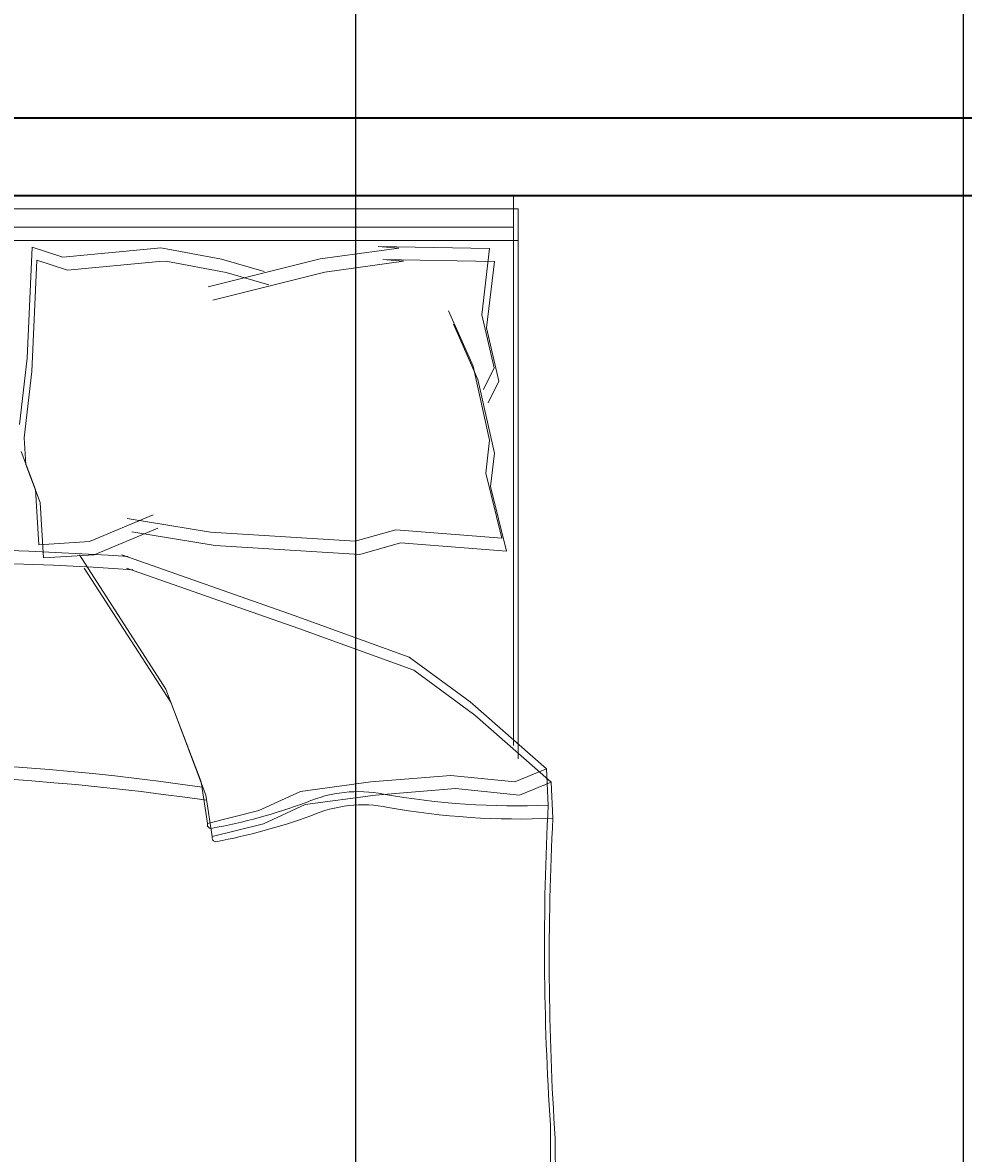
# Model space of a CAD drawing. Units: inches. Extents: x 1088 to 1703, y 668 to 1875.
# Tile 43 of 45: x 1531 to 1586, y 1743 to 1809. Entities that reach past the tile are written whole.
import ezdxf

# ---------------------------------------------------------------- set-up
doc = ezdxf.new("R2010")
doc.units = ezdxf.units.IN
for name, color, linetype, lineweight in [('A-ANNO-DIMS', 2, 'Continuous', 18), ('A-FURN', 8, 'Continuous', 13), ('A-WALL', 7, 'Continuous', 35)]:
    doc.layers.add(name, color=color, linetype=linetype, lineweight=lineweight)
doc.styles.get("Standard").update_dxf_attribs({"font": 'arial.ttf'})
doc.dimstyles.get("Standard").update_dxf_attribs({"dimtxt": 0.18, "dimasz": 0.18, "dimexe": 0.18, "dimexo": 0.0625, "dimgap": 0.09, "dimtad": 0, "dimtih": 1, "dimtoh": 1, "dimdec": 4, "dimzin": 0, "dimdsep": 46, "dimtxsty": 'Standard', "dimcen": 0.09, "dimadec": 0, "dimazin": 0, "dimtfac": 1, "dimtdec": 4, "dimtofl": 0, "dimtmove": 0, "dimatfit": 3, "dimfxl": 1, "dimtolj": 1, "dimtzin": 0, "dimarcsym": 0})

# ---------------------------------------------------------------- blocks, each defined once
blk = doc.blocks.new('BED-DOUBLE')
for p, q in [((34.03, 63.655), (30.133, 59.213)), ((36.121, 63.75), (34.03, 63.655, 4.641)), ((34.772, 61.812), (34.03, 63.655)), ((33.263, 63.381), (29.367, 58.939)), ((35.355, 63.476), (33.263, 63.381, 4.641)), ((34.006, 61.538), (33.263, 63.381)), ((0.766, 61.734), (32.668, 61.734)), ((0.766, 4.44), (0.766, 61.734)), ((2.605, 4.44), (2.605, 61.734)), ((34.401, 58.099), (34.772, 61.812)), ((0, 61.46), (31.901, 61.46)), ((0, 4.167), (0, 61.46)), ((1.838, 4.167), (1.838, 61.46)), ((20.635, 61.054), (16.872, 60.124)), ((20.151, 54.902), (20.635, 61.054)), ((33.634, 57.825), (34.006, 61.538)), ((3.832, 60.351), (3.716, 53.875)), ((3.832, 60.351), (7.681, 59.897)), ((7.681, 59.897), (10.763, 60.611)), ((14.947, 60.351), (10.665, 59.389)), ((10.763, 60.611), (12.017, 59.995)), ((16.872, 60.124), (14.947, 60.351)), ((19.868, 60.78), (16.105, 59.851)), ((19.384, 54.628), (19.868, 60.78)), ((3.065, 60.077), (2.949, 53.601)), ((3.065, 60.077), (6.915, 59.624)), ((6.915, 59.624), (9.996, 60.337)), ((14.181, 60.078), (9.899, 59.115)), ((9.996, 60.337), (11.251, 59.721)), ((16.105, 59.851), (14.181, 60.078)), ((9.899, 59.115), (6.688, 57.699)), ((10.665, 59.389), (7.454, 57.973)), ((30.133, 59.213), (27.535, 55.685)), ((29.367, 58.939), (26.769, 55.411)), ((34.006, 53.183), (33.634, 57.825)), ((34.772, 53.457), (34.401, 58.099)), ((26.769, 55.411), (24.357, 48.727)), ((27.535, 55.685), (25.123, 49.001)), ((2.949, 53.601), (3.048, 54.803)), ((3.048, 54.803), (3.68, 50.25)), ((3.716, 53.875), (3.814, 55.077)), ((3.814, 55.077), (4.446, 50.523)), ((20.052, 52.278), (19.384, 54.628)), ((20.819, 52.552), (20.151, 54.902)), ((34.562, 49.098), (34.006, 53.183)), ((35.329, 49.372), (34.772, 53.457)), ((20.302, 44.148), (20.819, 52.552)), ((19.536, 43.874), (20.052, 52.278)), ((4.446, 50.523), (6.068, 44.027)), ((3.68, 50.25), (5.301, 43.753)), ((36.442, 46.958), (35.329, 49.372)), ((24.357, 48.727), (20.84, 38.731)), ((25.123, 49.001), (21.606, 39.005)), ((35.676, 46.685), (34.562, 49.098)), ((5.171, 47.27), (4.457, 44.794)), ((4.404, 46.996), (3.69, 44.52)), ((36.418, 43.714), (35.676, 46.685)), ((37.184, 43.988), (36.442, 46.958)), ((4.457, 44.794), (3.808, 41.281)), ((3.69, 44.52), (3.042, 41.007)), ((19.503, 39.314), (20.302, 44.148)), ((34.772, 43.616), (37.184, 43.988)), ((18.736, 39.04), (19.536, 43.874)), ((28.624, 41.3), (34.006, 43.342)), ((29.391, 41.574), (34.772, 43.616)), ((34.006, 43.342), (36.418, 43.714)), ((21.606, 36.551), (29.391, 41.574)), ((3.042, 41.007), (3.066, 40.622)), ((3.808, 41.281), (3.832, 40.896)), ((3.832, 40.896), (4.338, 35.587)), ((20.835, 37.139), (19.294, 40.82)), ((20.84, 36.277), (28.624, 41.3)), ((3.066, 40.622), (3.571, 35.314)), ((20.068, 36.866), (18.528, 40.547)), ((20.252, 33.925), (20.068, 36.866)), ((21.018, 34.199), (20.835, 37.139)), ((4.338, 35.587), (3.754, 33.814)), ((3.571, 35.314), (2.987, 33.541)), ((17.81, 33.998), (21.018, 34.199)), ((2.987, 33.541), (9.432, 33.249)), ((3.754, 33.814), (10.198, 33.523)), ((10.198, 33.523), (14.047, 33.069)), ((14.838, 32.892), (17.044, 33.725)), ((15.604, 33.166), (17.81, 33.998)), ((17.044, 33.725), (20.252, 33.925)), ((9.432, 33.249), (13.281, 32.795)), ((14.047, 33.069), (15.604, 33.166))]:
    blk.add_line(p, q)
for centre, radius, start, end in [((-7.213, 61.808), 43.378, 349.87628, 2.56571), ((44.303, 218.785), 155.251, 266.97912, 273.83645), ((81.308, -5405.342), 5469.019, 90.002168, 90.286887), ((82.075, -5405.068), 5469.019, 90.002168, 90.286887), ((-7.98, 61.534), 43.378, 349.87628, 2.56571), ((43.537, 218.511), 155.251, 266.97912, 273.83645), ((42.039, 52.443), 7.462, 168.6608, 203.73842), ((42.806, 52.716), 7.462, 168.6608, 203.73842), ((1.777, 37.349), 35.551, 10.66171, 19.88058), ((2.543, 37.623), 35.551, 10.66171, 19.88058), ((37.259, 44.196), 0.221, 250.24637, 1.13765), ((187.401, 21.287), 154.676, 171.78449, 186.90062), ((188.167, 21.561), 154.676, 171.78449, 186.90062), ((36.492, 43.922), 0.221, 250.24637, 1.13765), ((219.021, 25.88), 197.774, 176.08655, 186.78213), ((218.255, 25.607), 197.774, 176.08655, 186.78213)]:
    blk.add_arc(centre, radius, start, end)
blk = doc.blocks.new('*D28')
at = {"layer": 'A-ANNO-DIMS', "color": 0, "lineweight": -2, "transparency": 16777216}
for p, q in [((1170.345, 1803.621), (1170.345, 1857.788)), ((1170.525, 1857.608), (1408.147, 1857.608)), ((1646.563, 1857.608), (1408.941, 1857.608)), ((1646.743, 1745.552), (1646.743, 1857.788))]:
    blk.add_line(p, q, dxfattribs=at)
at = {"layer": 'A-ANNO-DIMS', "color": 0, "transparency": 16777216}
for points in [[(1170.525, 1857.638), (1170.525, 1857.578), (1170.345, 1857.608)], [(1646.563, 1857.638), (1646.563, 1857.578), (1646.743, 1857.608)]]:
    blk.add_solid(points, dxfattribs=at)
at = {"layer": 'Defpoints', "color": 0, "transparency": 16777216}
for p in [(1646.743, 1857.608), (1170.345, 1803.558), (1646.743, 1745.49)]:
    blk.add_point(p, dxfattribs=at)
at = {"layer": 'A-ANNO-DIMS', "color": 0, "transparency": 16777216, "insert": (1408.544, 1857.608), "char_height": 0.18, "attachment_point": 5}
blk.add_mtext('\\A1;476.4', dxfattribs=at)
blk = doc.blocks.new('*D32')
at = {"layer": 'A-ANNO-DIMS', "color": 0, "lineweight": -2, "transparency": 16777216}
for p, q in [((1550.595, 1373.121), (1550.595, 1857.788)), ((1550.775, 1857.608), (1567.825, 1857.608)), ((1585.665, 1857.608), (1568.614, 1857.608)), ((1585.845, 1360.983), (1585.845, 1857.788))]:
    blk.add_line(p, q, dxfattribs=at)
at = {"layer": 'A-ANNO-DIMS', "color": 0, "transparency": 16777216}
for points in [[(1550.775, 1857.638), (1550.775, 1857.578), (1550.595, 1857.608)], [(1585.665, 1857.638), (1585.665, 1857.578), (1585.845, 1857.608)]]:
    blk.add_solid(points, dxfattribs=at)
at = {"layer": 'Defpoints', "color": 0, "transparency": 16777216}
for p in [(1585.845, 1857.608), (1550.595, 1373.058), (1585.845, 1360.921)]:
    blk.add_point(p, dxfattribs=at)
at = {"layer": 'A-ANNO-DIMS', "color": 0, "transparency": 16777216, "insert": (1568.22, 1857.608), "char_height": 0.18, "attachment_point": 5}
blk.add_mtext('\\A1;35.25', dxfattribs=at)

msp = doc.modelspace()

# ---------------------------------------------------------------- linework, layer by layer
at = {"layer": 'A-WALL'}
for p, q in [((1437.345, 1803.558), (1624.845, 1803.558)), ((1437.345, 1803.558), (1624.845, 1803.558)), ((1437.345, 1803.558), (1624.845, 1803.558)), ((1437.345, 1803.558), (1624.845, 1803.558)), ((1437.345, 1803.558), (1624.845, 1803.558)), ((1441.845, 1799.058), (1620.345, 1799.058))]:
    msp.add_line(p, q, dxfattribs=at)

# ---------------------------------------------------------------- block references
at = {"layer": 'A-FURN', "rotation": 270}
msp.add_blockref('BED-DOUBLE', (1498.281, 1799.058), dxfattribs=at)

# ---------------------------------------------------------------- dimensions: what is measured, and where the dimension line sits
at = {"layer": 'A-ANNO-DIMS'}
for base, p1, p2, override, picture, middle in [((1646.743, 1857.608), (1170.345, 1803.558), (1646.743, 1745.49), {"dimdec": 1, "dimlfac": 1, "dimrnd": 0, "dimzin": 0, "dimdsep": 46, "dimlunit": 2}, '*D28', (1408.544, 1857.608)), ((1585.845, 1857.608), (1550.595, 1373.058), (1585.845, 1360.921), {"dimdec": 2, "dimlfac": 1, "dimrnd": 0, "dimzin": 0, "dimdsep": 46, "dimlunit": 2}, '*D32', (1568.22, 1857.608))]:
    dim = msp.add_linear_dim(base=base, p1=p1, p2=p2, dimstyle='Standard', override=override, dxfattribs=at)
    dim.commit()
    dim.dimension.update_dxf_attribs({"geometry": picture, "text_midpoint": middle})

doc.saveas('drawing.dxf')
